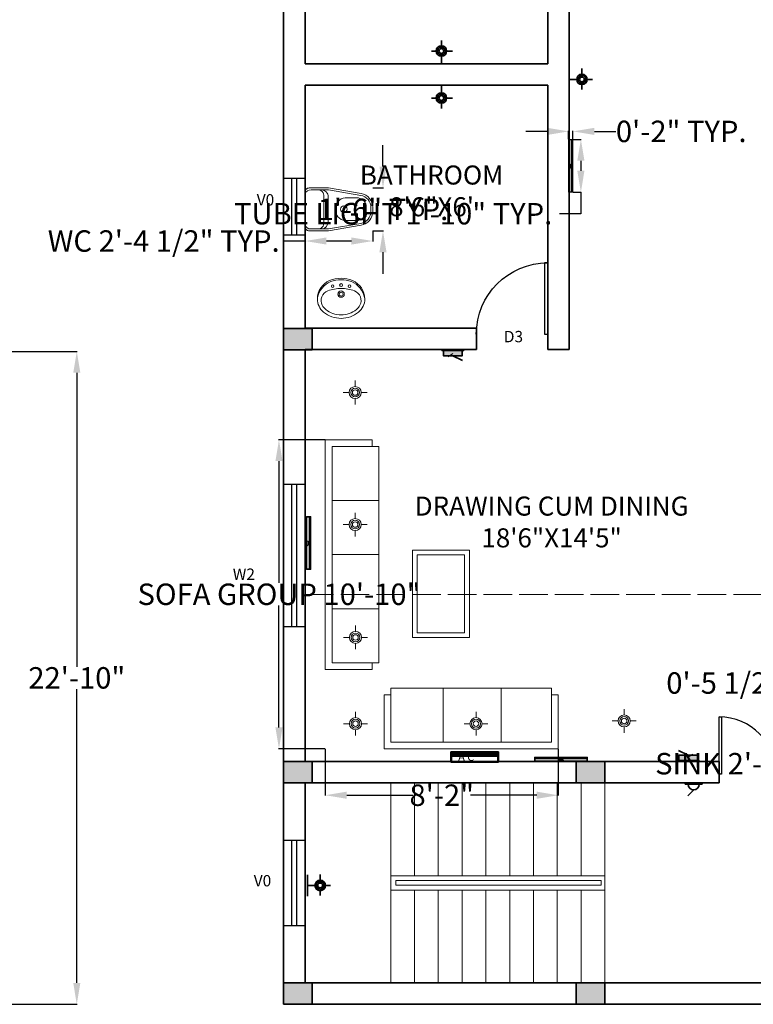
# Model space of a CAD drawing. Units: inches. Extents: x 68 to 1275, y 90 to 1276.
# Tile 4 of 6: x 608 to 916, y 603 to 1017. Entities that reach past the tile are written whole.
import ezdxf

# ---------------------------------------------------------------- set-up
doc = ezdxf.new("R2010")
doc.units = ezdxf.units.IN
doc.header["$MEASUREMENT"] = 0
doc.linetypes.add('ACAD_ISO02W100', pattern=[15, 12, -3])
for name, color, linetype, lineweight in [('A -Elec', 6, 'Continuous', 18), ('A-ANNO-TEXT', 7, 'Continuous', 18), ('A-AREA-IDEN', 7, 'Continuous', 18), ('A-FLOR-FIXT', 9, 'Continuous', 18), ('A-FURN', 150, 'Continuous', 5), ('A-WALL', 7, 'Continuous', 35), ('COLUMN', 150, 'Continuous', 35), ('DIM', 2, 'Continuous', 18), ('DOOR', 15, 'Continuous', 25), ('E-EQPM', 1, 'Continuous', 18), ('E-LITE', 6, 'Continuous', 18), ('E-POWR', 1, 'Continuous', 18), ('E-REFR', 8, 'ACAD_ISO02W100', 13), ('Elec', 1, 'Continuous', 35), ('FURN', 163, 'Continuous', 18), ('STAIRCASE', 40, 'Continuous', 18), ('WINDOW', 17, 'Continuous', 18)]:
    doc.layers.add(name, color=color, linetype=linetype, lineweight=lineweight)
doc.styles.get("Standard").update_dxf_attribs({"font": 'arial.ttf'})
doc.dimstyles.get("Standard").update_dxf_attribs({"dimtxt": 9, "dimasz": 9, "dimexe": 0.18, "dimexo": 0.0625, "dimgap": 0.09, "dimtad": 0, "dimtih": 1, "dimtoh": 1, "dimdec": 1, "dimzin": 0, "dimdsep": 46, "dimlunit": 3, "dimtxsty": 'Standard', "dimcen": 0.09, "dimadec": 0, "dimazin": 0, "dimtfac": 1, "dimtdec": 1, "dimtofl": 0, "dimtmove": 0, "dimatfit": 3, "dimfxl": 1, "dimtolj": 1, "dimtzin": 0, "dimarcsym": 0})

# ---------------------------------------------------------------- blocks, each defined once
blk = doc.blocks.new('*U2')
for p, q in [((0, 0), (0, -6)), ((40, 0), (40, -6))]:
    blk.add_line(p, q)
blk.add_lwpolyline([(0, 0), (0, 40), (1.75, 40), (1.75, 0)], close=True)
blk.add_arc((0, 0), 40, 0, 90)
blk = doc.blocks.new('W')
at = {"layer": 'DOOR'}
for p, q in [((91.84, 414.95), (100.84, 414.95)), ((91.84, 354.95), (91.84, 414.95)), ((95.34, 354.95), (95.34, 414.95)), ((97.34, 354.95), (97.34, 414.95)), ((100.84, 414.95), (100.84, 354.95)), ((100.84, 354.95), (91.84, 354.95))]:
    blk.add_line(p, q, dxfattribs=at)
blk = doc.blocks.new('V')
at = {"layer": 'DOOR'}
for p, q in [((554.81, 674.59), (563.81, 674.59)), ((554.81, 650.59), (554.81, 674.59)), ((558.31, 650.59), (558.31, 674.59)), ((560.31, 650.59), (560.31, 674.59)), ((563.81, 674.59), (563.81, 650.59)), ((563.81, 650.59), (554.81, 650.59))]:
    blk.add_line(p, q, dxfattribs=at)
blk = doc.blocks.new('W2')
at = {"layer": 'DOOR'}
for p, q in [((130.85, 208.71), (130.85, 244.71)), ((130.85, 244.71), (139.85, 244.71)), ((134.35, 208.71), (134.35, 244.71)), ((136.35, 208.71), (136.35, 244.71)), ((139.85, 244.71), (139.85, 208.71)), ((139.85, 208.71), (130.85, 208.71))]:
    blk.add_line(p, q, dxfattribs=at)
blk = doc.blocks.new('C')
h = blk.add_hatch(color=256)
h.dxf.hatch_style = 1
h.paths.add_polyline_path([(745.81, 845.98), (745.81, 857.98), (736.81, 857.98), (736.81, 845.98)])
for p, q in [((745.81, 857.98), (736.81, 857.98)), ((736.81, 857.98), (736.81, 845.98)), ((745.81, 845.98), (745.81, 857.98)), ((736.81, 845.98), (745.81, 845.98))]:
    blk.add_line(p, q)
blk = doc.blocks.new('SOFA')
at = {"layer": 'FURN'}
for p, q in [((2092.6, 1660), (2069.89, 1660)), ((2092.6, 1635.73), (2069.89, 1635.73)), ((1991.15, 1608.68), (1991.15, 1588.96)), ((2013.86, 1608.68), (2013.86, 1588.96)), ((2036.57, 1608.68), (2036.57, 1588.96))]:
    blk.add_line(p, q, dxfattribs=at)
for points in [[(2072.73, 1681.16), (2072.73, 1684), (2095.44, 1684), (2095.44, 1610.84), (2072.73, 1610.84), (2072.73, 1613.68)], [(1968.43, 1605.84), (1965.59, 1605.84), (1965.59, 1586.12), (2062.13, 1586.12), (2062.13, 1605.84), (2059.29, 1605.84)]]:
    blk.add_lwpolyline(points, dxfattribs=at)
for points in [[(2092.6, 1681.16), (2092.6, 1613.68), (2069.89, 1613.68), (2069.89, 1681.16)], [(1968.43, 1588.96), (2059.29, 1588.96), (2059.29, 1608.68), (1968.43, 1608.68)]]:
    blk.add_lwpolyline(points, close=True, dxfattribs=at)
blk = doc.blocks.new('WC')
at = {"layer": 'A-FURN'}
for p, q in [((171114.18, -56009.21), (171100.52, -56011.54)), ((171114.18, -56009.21), (171122.29, -56009.21)), ((171124.07, -56010.99), (171124.07, -56025.42)), ((171095.59, -56017.39), (171095.59, -56019.02)), ((171114.18, -56027.21), (171100.52, -56024.87)), ((171122.29, -56027.21), (171114.18, -56027.21))]:
    blk.add_line(p, q, dxfattribs=at)
for points in [[(171114.18, -56027.21), (171122.29, -56027.21, 0.414214), (171124.07, -56025.42), (171124.07, -56010.99, 0.414214), (171122.29, -56009.21), (171114.18, -56009.21), (171100.52, -56011.54, 0.365402), (171095.59, -56017.39), (171095.59, -56019.02, 0.365402), (171100.52, -56024.87)], [(171114.25, -56026.41), (171121.5, -56026.41, 0.361508), (171124.07, -56024.7), (171124.07, -56011.71, 0.375474), (171121.68, -56010), (171114.25, -56010), (171100.66, -56012.32, 0.365402), (171096.38, -56017.39), (171096.38, -56019.02, 0.365402), (171100.66, -56024.09)], [(171124.07, -56011.71), (171124.07, -56024.7, -0.361508), (171121.5, -56026.41), (171117.23, -56026.41, -0.430105), (171114.38, -56023.46), (171114.38, -56012.95, -0.411531), (171117.23, -56010), (171121.68, -56010, -0.375474)], [(171124.07, -56011.71), (171124.07, -56024.7, -0.361508), (171121.5, -56026.41), (171118.83, -56026.41, -0.480412), (171116.16, -56023.63), (171116.16, -56012.78, -0.482705), (171118.83, -56010), (171121.68, -56010, -0.375474)], [(171106.42, -56023.02, 0.46477), (171111.04, -56019.12), (171111.04, -56017.49, 0.46477), (171106.42, -56013.59), (171101.64, -56013.59, 0.365402), (171098.35, -56017.49), (171098.35, -56019.12, 0.365402), (171101.64, -56023.02)], [(171107.8, -56016.9, -1), (171107.8, -56019.71, -1)]]:
    blk.add_lwpolyline(points, format="xyb", close=True, dxfattribs=at)
for centre, radius, start, end in [((171101.52, -56017.39), 5.93, 99.7106, 180.0002), ((171122.29, -56010.99), 1.78, 0.0002, 90.0002), ((171101.52, -56019.02), 5.93, 180.0002, 260.2897), ((171122.29, -56025.42), 1.78, 270.0002, 0.0002)]:
    blk.add_arc(centre, radius, start, end, dxfattribs=at)
blk = doc.blocks.new('Basin')
at = {"layer": 'A-FURN'}
for centre, radius in [((171010.96, -56068.51), 0.593), ((171010.45, -56072.47), 0.692), ((171014.68, -56072.47), 1.48), ((171014.68, -56072.47), 0.91), ((171010.96, -56076.42), 0.593)]:
    blk.add_circle(centre, radius, dxfattribs=at)
for centre, radius, start, end in [((171018.29, -56073.43), 10.2, 262.5047, 262.5047), ((171016.96, -56070.69), 9.3, 90, 157.2856), ((171018.29, -56071.51), 10.2, 100.9967, 157.8207), ((171017.65, -56067.95), 4.81, 62.931, 159.6415), ((171016.96, -56069.3), 7.91, 39.0829, 90), ((171016.96, -56069.3), 6.33, 39.0829, 62.931), ((171013.06, -56072.47), 12.93, 0, 39.0829), ((171021.21, -56072.47), 13.91, 157.2856, 180), ((171021.21, -56072.47), 13.27, 158.7467, 180), ((171029.84, -56072.47), 17.8, 159.6415, 180), ((171013.06, -56072.47), 11.35, 0, 39.0829), ((171021.21, -56072.47), 13.91, 180, 202.7144), ((171021.21, -56072.47), 13.27, 180, 201.2533), ((171029.84, -56072.47), 17.8, 180, 200.3585), ((171013.06, -56072.47), 11.35, 320.9171, 0), ((171013.06, -56072.47), 12.93, 320.9171, 0), ((171016.96, -56074.25), 9.3, 202.7144, 270), ((171018.29, -56073.43), 10.2, 202.1793, 259.0033), ((171017.65, -56076.99), 4.81, 200.3585, 297.069), ((171016.96, -56075.63), 7.91, 270, 320.9171), ((171016.96, -56075.63), 6.33, 297.069, 320.9171)]:
    blk.add_arc(centre, radius, start, end, dxfattribs=at)
blk = doc.blocks.new('splight')
at = {"layer": 'Elec'}
for p, q in [((4618.17, 527.16), (4627.57, 527.16)), ((4622.87, 527.16), (4622.87, 523.87)), ((4620.58, 521.58), (4618.05, 521.58)), ((4625.16, 521.58), (4627.23, 521.58)), ((4622.87, 519.28), (4622.87, 517.03))]:
    blk.add_line(p, q, dxfattribs=at)
for radius in [2.29, 1.67, 1.04]:
    blk.add_circle((4622.87, 521.58), radius, dxfattribs=at)
blk = doc.blocks.new('tube')
at = {"layer": 'A -Elec'}
for p, q in [((4592.61, 556.75), (4641.61, 556.75)), ((4592.61, 555.25), (4592.61, 556.75)), ((4593.11, 555.25), (4593.11, 556.75)), ((4593.11, 556.33), (4593.41, 556.33)), ((4593.41, 555.25), (4593.41, 556.75)), ((4593.41, 556.5), (4640.81, 556.5)), ((4640.81, 555.25), (4640.81, 556.75)), ((4640.81, 556.33), (4641.11, 556.33)), ((4641.11, 556.75), (4641.11, 555.25)), ((4641.11, 555.25), (4641.11, 556.75)), ((4641.61, 556.75), (4641.61, 555.25)), ((4592.61, 552.75), (4592.61, 555.25)), ((4592.61, 552.75), (4641.61, 552.75)), ((4593.11, 556.21), (4593.41, 556.21)), ((4593.11, 555.81), (4593.41, 555.81)), ((4593.11, 555.69), (4593.41, 555.69)), ((4641.11, 555.25), (4593.11, 555.25)), ((4593.11, 555.25), (4593.11, 553.25)), ((4593.11, 553.25), (4593.11, 555.25)), ((4593.11, 553.25), (4641.61, 553.25)), ((4593.41, 556.25), (4640.81, 556.25)), ((4593.41, 556), (4640.81, 556)), ((4593.41, 555.75), (4640.81, 555.75)), ((4593.41, 555.5), (4640.81, 555.5)), ((4640.81, 556.21), (4641.11, 556.21)), ((4640.81, 555.81), (4641.11, 555.81)), ((4640.81, 555.69), (4641.11, 555.69)), ((4641.11, 553.25), (4641.11, 555.25)), ((4641.61, 552.75), (4641.61, 555.25))]:
    blk.add_line(p, q, dxfattribs=at)
for points in [[(4615.6, 553.25), (4619.11, 553.25), (4619.11, 554.31), (4615.6, 554.31)], [(4619.11, 553.78), (4619.11, 553.78), (4619.11, 553.78), (4619.11, 553.78)], [(4619.11, 553.78), (4619.81, 553.78), (4619.81, 553.25), (4619.11, 553.25)]]:
    blk.add_lwpolyline(points, close=True, dxfattribs=at)
blk = doc.blocks.new('CIELING')
at = {"layer": 'A -Elec'}
for p, q in [((1070.87, -8395.66), (1070.87, -8391.49)), ((1066.61, -8399.91), (1062.44, -8399.91)), ((1075.13, -8399.91), (1079.29, -8399.91)), ((1070.87, -8408.34), (1070.87, -8404.17))]:
    blk.add_line(p, q, dxfattribs=at)
for radius in [4.26, 3.1, 1.94]:
    blk.add_circle((1070.87, -8399.91), radius, dxfattribs=at)
blk = doc.blocks.new('BELL SWITCH')
at = {"layer": 'Elec'}
for p, q in [((4981.81, 3401.31), (4981.81, 3402.27)), ((4981.81, 3402.27), (4993.57, 3402.27)), ((4993.57, 3402.27), (4993.57, 3401.31)), ((4993.57, 3401.31), (4981.81, 3401.31)), ((4987.69, 3397.36), (4983.52, 3393.3))]:
    blk.add_line(p, q, dxfattribs=at)
blk.add_arc((4987.69, 3401.31), 3.95, 180, 0, dxfattribs=at)
blk = doc.blocks.new('ac')
at = {"layer": 'Elec'}
for p, q in [((12718.34, -53.78), (12674.36, -53.78)), ((12674.36, -63.02), (12674.36, -53.78)), ((12675.81, -57.52), (12675.81, -53.78)), ((12717.03, -57.52), (12717.03, -53.78)), ((12718.34, -63.02), (12718.34, -53.78)), ((12718.34, -63.02), (12674.36, -63.02)), ((12674.89, -57.52), (12717.81, -57.52)), ((12717.03, -54.85), (12675.81, -54.85)), ((12717.03, -56.21), (12675.81, -56.21))]:
    blk.add_line(p, q, dxfattribs=at)
at = {"layer": 'Elec', "ltscale": 0.1}
for p, q in [((12674.89, -61.49), (12674.89, -53.78)), ((12717.03, -54.36), (12675.81, -54.36)), ((12717.81, -61.49), (12717.81, -53.78)), ((12717.03, -55.66), (12675.81, -55.66)), ((12717.03, -56.84), (12675.81, -56.84)), ((12716.81, -62.49), (12675.89, -62.49))]:
    blk.add_line(p, q, dxfattribs=at)
at = {"layer": 'Elec'}
for centre, start, end in [((12675.89, -61.49), 180, 270), ((12716.81, -61.49), 270, 0)]:
    blk.add_arc(centre, 1, start, end, dxfattribs=at)
blk = doc.blocks.new('STAIR-RETURN-PLAN')
for p, q in [((0, 84), (0, 0)), ((10, 84), (10, 45)), ((20, 84), (20, 45)), ((30, 84), (30, 45)), ((40, 84), (40, 45)), ((50, 84), (50, 45)), ((60, 84), (60, 45)), ((70, 84), (70, 45)), ((80, 84), (80, 45)), ((90, 84), (90, 0)), ((0, 45), (90, 45)), ((2.15, 43), (88.44, 43)), ((2.15, 41), (2.15, 43)), ((88.44, 41), (88.44, 43)), ((0, 39), (90, 39)), ((2.15, 41), (88.44, 41)), ((10, 39), (10, 0)), ((20, 39), (20, 0)), ((30, 39), (30, 0)), ((40, 39), (40, 0)), ((50, 39), (50, 0)), ((60, 39), (60, 0)), ((70, 39), (70, 0)), ((80, 39), (80, 0))]:
    blk.add_line(p, q)
blk = doc.blocks.new('elec box')
at = {"layer": 'Elec'}
blk.add_hatch(color=256, dxfattribs=at).paths.add_polyline_path([(3828.23, 599.29), (3828.23, 594.79), (3844.73, 594.79), (3844.73, 599.29)])
for p, q in [((3836.48, 599.29), (3828.07, 603.45)), ((3846.1, 594.79), (3826.83, 594.79)), ((3826.83, 594.79), (3826.83, 593.89)), ((3846.1, 593.89), (3846.1, 594.79)), ((3826.83, 593.89), (3846.1, 593.89))]:
    blk.add_line(p, q, dxfattribs=at)
blk.add_lwpolyline([(3828.23, 594.79), (3828.23, 599.29), (3844.73, 599.29), (3844.73, 594.79), (3828.23, 594.79)], dxfattribs=at)
blk = doc.blocks.new('SWITCHBOARD-ONE-WAY')
blk.add_line((4.63, 1.73), (6.64, 3.12))
at = {"xscale": 0.480395109260985, "yscale": 0.480395109260985, "zscale": 0.480395109260985}
blk.add_blockref('elec box', (-1838.39, -285.3), dxfattribs=at)
blk = doc.blocks.new('*D59')
at = {"layer": 'Defpoints', "color": 0, "transparency": 16777216}
for p in [(727.63, 928.31), (756.11, 928.31), (727.63, 924.04)]:
    blk.add_point(p, dxfattribs=at)
at = {"layer": 'DIM', "color": 0, "lineweight": -2, "transparency": 16777216}
for p, q in [((727.63, 928.25), (727.63, 923.86)), ((756.11, 928.25), (756.11, 923.86)), ((727.63, 924.04), (718.63, 924.04)), ((747.11, 924.04), (736.63, 924.04))]:
    blk.add_line(p, q, dxfattribs=at)
at = {"layer": 'DIM', "color": 0, "transparency": 16777216}
for points in [[(736.63, 925.54), (736.63, 922.54), (727.63, 924.04)], [(747.11, 925.54), (747.11, 922.54), (756.11, 924.04)]]:
    blk.add_solid(points, dxfattribs=at)
at = {"layer": 'DIM', "color": 0, "transparency": 16777216, "insert": (668.22, 924.04), "char_height": 9, "attachment_point": 5}
blk.add_mtext('\\A1;WC 2\'-4 1/2" TYP.', dxfattribs=at)
blk = doc.blocks.new('*D60')
at = {"layer": 'Defpoints', "color": 0, "transparency": 16777216}
for p in [(756.11, 946.31), (756.11, 928.31), (760.38, 928.31)]:
    blk.add_point(p, dxfattribs=at)
at = {"layer": 'DIM', "color": 0, "lineweight": -2, "transparency": 16777216}
for p, q in [((760.38, 955.31), (760.38, 964.31)), ((756.17, 946.31), (760.56, 946.31)), ((756.17, 928.31), (760.56, 928.31)), ((760.38, 919.31), (760.38, 910.31))]:
    blk.add_line(p, q, dxfattribs=at)
at = {"layer": 'DIM', "color": 0, "transparency": 16777216}
for points in [[(758.88, 955.31), (761.88, 955.31), (760.38, 946.31)], [(758.88, 919.31), (761.88, 919.31), (760.38, 928.31)]]:
    blk.add_solid(points, dxfattribs=at)
at = {"layer": 'DIM', "color": 0, "transparency": 16777216, "insert": (760.38, 937.31), "char_height": 9, "attachment_point": 5}
blk.add_mtext('\\A1;1\'-6" TYP.', dxfattribs=at)
blk = doc.blocks.new('*D63')
at = {"layer": 'Defpoints', "color": 0, "transparency": 16777216}
for p in [(736.14, 840.6), (716.66, 710.75), (736.14, 710.75)]:
    blk.add_point(p, dxfattribs=at)
at = {"layer": 'DIM', "color": 0, "lineweight": -2, "transparency": 16777216}
for p, q in [((736.07, 840.6), (716.48, 840.6)), ((716.66, 831.6), (716.66, 780.43)), ((716.66, 719.75), (716.66, 770.93)), ((736.07, 710.75), (716.48, 710.75))]:
    blk.add_line(p, q, dxfattribs=at)
at = {"layer": 'DIM', "color": 0, "transparency": 16777216}
for points in [[(715.16, 831.6), (718.16, 831.6), (716.66, 840.6)], [(715.16, 719.75), (718.16, 719.75), (716.66, 710.75)]]:
    blk.add_solid(points, dxfattribs=at)
at = {"layer": 'DIM', "color": 0, "transparency": 16777216, "insert": (716.66, 775.68), "char_height": 9, "attachment_point": 5}
blk.add_mtext('\\A1;SOFA GROUP 10\'-10"', dxfattribs=at)
blk = doc.blocks.new('*D64')
at = {"layer": 'Defpoints', "color": 0, "transparency": 16777216}
for p in [(736.14, 710.75), (834.01, 710.75), (834.01, 691.28)]:
    blk.add_point(p, dxfattribs=at)
at = {"layer": 'DIM', "color": 0, "lineweight": -2, "transparency": 16777216}
for p, q in [((736.14, 710.69), (736.14, 691.1)), ((834.01, 710.69), (834.01, 691.1)), ((745.14, 691.28), (773.02, 691.28)), ((825.01, 691.28), (797.13, 691.28))]:
    blk.add_line(p, q, dxfattribs=at)
at = {"layer": 'DIM', "color": 0, "transparency": 16777216}
for points in [[(745.14, 692.78), (745.14, 689.78), (736.14, 691.28)], [(825.01, 692.78), (825.01, 689.78), (834.01, 691.28)]]:
    blk.add_solid(points, dxfattribs=at)
at = {"layer": 'DIM', "color": 0, "transparency": 16777216, "insert": (785.08, 691.28), "char_height": 9, "attachment_point": 5}
blk.add_mtext('\\A1;8\'-2"', dxfattribs=at)
blk = doc.blocks.new('*D68')
at = {"layer": 'Defpoints', "color": 0, "transparency": 16777216}
for p in [(944.14, 747.41), (949.63, 747.41), (944.14, 738.41)]:
    blk.add_point(p, dxfattribs=at)
at = {"layer": 'DIM', "color": 0, "lineweight": -2, "transparency": 16777216}
for p, q in [((944.14, 747.35), (944.14, 738.23)), ((949.63, 747.35), (949.63, 738.23)), ((935.14, 738.41), (926.14, 738.41)), ((958.63, 738.41), (967.63, 738.41))]:
    blk.add_line(p, q, dxfattribs=at)
at = {"layer": 'DIM', "color": 0, "transparency": 16777216}
for points in [[(935.14, 739.91), (935.14, 736.91), (944.14, 738.41)], [(958.63, 739.91), (958.63, 736.91), (949.63, 738.41)]]:
    blk.add_solid(points, dxfattribs=at)
at = {"layer": 'DIM', "color": 0, "transparency": 16777216, "insert": (903.6, 738.41), "char_height": 9, "attachment_point": 5}
blk.add_mtext('\\A1;0\'-5 1/2"', dxfattribs=at)
blk = doc.blocks.new('*D69')
at = {"layer": 'Defpoints', "color": 0, "transparency": 16777216}
for p in [(962.08, 709.07), (992.43, 709.07), (962.08, 704.52)]:
    blk.add_point(p, dxfattribs=at)
at = {"layer": 'DIM', "color": 0, "lineweight": -2, "transparency": 16777216}
for p, q in [((962.08, 709.01), (962.08, 704.34)), ((992.43, 709.01), (992.43, 704.34)), ((962.08, 704.52), (953.08, 704.52)), ((983.43, 704.52), (971.08, 704.52))]:
    blk.add_line(p, q, dxfattribs=at)
at = {"layer": 'DIM', "color": 0, "transparency": 16777216}
for points in [[(971.08, 706.02), (971.08, 703.02), (962.08, 704.52)], [(983.43, 706.02), (983.43, 703.02), (992.43, 704.52)]]:
    blk.add_solid(points, dxfattribs=at)
at = {"layer": 'DIM', "color": 0, "transparency": 16777216, "insert": (914.15, 704.52), "char_height": 9, "attachment_point": 5}
blk.add_mtext('\\A1;SINK 2\'-6 1/2"', dxfattribs=at)
blk = doc.blocks.new('*D75')
at = {"layer": 'Defpoints', "color": 0, "transparency": 16777216}
for p in [(840.21, 966.74), (840.21, 944.52), (843.55, 944.52)]:
    blk.add_point(p, dxfattribs=at)
at = {"layer": 'DIM', "color": 0, "lineweight": -2, "transparency": 16777216}
for p, q in [((840.28, 966.74), (843.73, 966.74)), ((843.55, 957.74), (843.55, 953.52)), ((840.28, 944.52), (843.73, 944.52)), ((843.55, 944.52), (843.55, 935.52)), ((843.55, 935.52), (834.55, 935.52))]:
    blk.add_line(p, q, dxfattribs=at)
at = {"layer": 'DIM', "color": 0, "transparency": 16777216}
for points in [[(842.05, 957.74), (845.05, 957.74), (843.55, 966.74)], [(842.05, 953.52), (845.05, 953.52), (843.55, 944.52)]]:
    blk.add_solid(points, dxfattribs=at)
at = {"layer": 'DIM', "color": 0, "transparency": 16777216, "insert": (764.65, 935.52), "char_height": 9, "attachment_point": 5}
blk.add_mtext('\\A1;TUBE LIGHT 1\'-10" TYP.', dxfattribs=at)
blk = doc.blocks.new('*D76')
at = {"layer": 'Defpoints', "color": 0, "transparency": 16777216}
for p in [(840.21, 970.08), (838.4, 966.74), (840.21, 966.74)]:
    blk.add_point(p, dxfattribs=at)
at = {"layer": 'DIM', "color": 0, "lineweight": -2, "transparency": 16777216}
for p, q in [((829.4, 970.08), (820.4, 970.08)), ((838.4, 966.81), (838.4, 970.26)), ((840.21, 966.81), (840.21, 970.26)), ((849.21, 970.08), (858.21, 970.08))]:
    blk.add_line(p, q, dxfattribs=at)
at = {"layer": 'DIM', "color": 0, "transparency": 16777216}
for points in [[(829.4, 971.58), (829.4, 968.58), (838.4, 970.08)], [(849.21, 971.58), (849.21, 968.58), (840.21, 970.08)]]:
    blk.add_solid(points, dxfattribs=at)
at = {"layer": 'DIM', "color": 0, "transparency": 16777216, "insert": (885.73, 970.08), "char_height": 9, "attachment_point": 5}
blk.add_mtext('\\A1;0\'-2" TYP.', dxfattribs=at)
blk = doc.blocks.new('*D84')
at = {"layer": 'Defpoints', "color": 0, "transparency": 16777216}
for p in [(594.19, 877.68), (631.69, 877.68), (534.19, 603.47)]:
    blk.add_point(p, dxfattribs=at)
at = {"layer": 'DIM', "color": 0, "lineweight": -2, "transparency": 16777216}
for p, q in [((594.25, 877.68), (631.87, 877.68)), ((631.69, 868.68), (631.69, 745.26)), ((631.69, 612.47), (631.69, 735.89)), ((534.25, 603.47), (631.87, 603.47))]:
    blk.add_line(p, q, dxfattribs=at)
at = {"layer": 'DIM', "color": 0, "transparency": 16777216}
for points in [[(630.19, 868.68), (633.19, 868.68), (631.69, 877.68)], [(630.19, 612.47), (633.19, 612.47), (631.69, 603.47)]]:
    blk.add_solid(points, dxfattribs=at)
at = {"layer": 'DIM', "color": 0, "transparency": 16777216, "insert": (631.69, 740.57), "char_height": 9, "attachment_point": 5}
blk.add_mtext('\\A1;22\'-10"', dxfattribs=at)
blk = doc.blocks.new('*D112')
at = {"layer": 'Defpoints', "color": 0, "transparency": 16777216}
for p in [(1147.63, 1270.42), (718.63, 1232.47), (1147.63, 988.68)]:
    blk.add_point(p, dxfattribs=at)
at = {"layer": 'DIM', "color": 0, "lineweight": -2, "transparency": 16777216}
for p, q in [((718.63, 1232.53), (718.63, 1270.6)), ((727.63, 1270.42), (917.58, 1270.42)), ((1138.63, 1270.42), (948.67, 1270.42)), ((1147.63, 988.74), (1147.63, 1270.6))]:
    blk.add_line(p, q, dxfattribs=at)
at = {"layer": 'DIM', "color": 0, "transparency": 16777216}
for points in [[(727.63, 1271.92), (727.63, 1268.92), (718.63, 1270.42)], [(1138.63, 1271.92), (1138.63, 1268.92), (1147.63, 1270.42)]]:
    blk.add_solid(points, dxfattribs=at)
at = {"layer": 'DIM', "color": 0, "transparency": 16777216, "insert": (933.13, 1270.42), "char_height": 9, "attachment_point": 5}
blk.add_mtext('\\A1;35\'-9"', dxfattribs=at)

msp = doc.modelspace()

# ---------------------------------------------------------------- linework, layer by layer
at = {"layer": 'A-WALL'}
for p, q in [((718.63, 1232.47), (718.63, 603.47)), ((727.63, 1082.47), (727.63, 998.47)), ((829.63, 1082.47), (829.63, 998.47)), ((838.63, 1082.47), (838.63, 986.47)), ((727.63, 998.47), (829.63, 998.47)), ((727.63, 989.47), (829.63, 989.47)), ((727.63, 989.47), (727.63, 887.47)), ((829.63, 989.47), (829.63, 887.47)), ((838.63, 986.47), (838.63, 878.47)), ((727.63, 887.47), (799.63, 887.47)), ((799.63, 887.47), (799.63, 878.47)), ((829.63, 887.47), (829.63, 878.47)), ((727.63, 878.47), (799.63, 878.47)), ((727.63, 878.47), (727.63, 705.47)), ((829.63, 878.47), (838.63, 878.47)), ((727.63, 705.47), (901.63, 705.47)), ((901.63, 696.47), (901.63, 705.47)), ((727.63, 696.47), (901.63, 696.47)), ((727.63, 696.47), (727.63, 612.47)), ((727.63, 612.47), (949.63, 612.47)), ((718.63, 603.47), (1087.63, 603.47))]:
    msp.add_line(p, q, dxfattribs=at)
at = {"layer": 'E-REFR'}
msp.add_line((727.63, 775.56), (949.63, 775.56), dxfattribs=at)
at = {"layer": 'FURN'}
for points in [[(796.69, 757.54), (772.77, 757.54), (772.77, 794.24), (796.69, 794.24)], [(794.69, 759.54), (774.77, 759.54), (774.77, 792.24), (794.69, 792.24)]]:
    msp.add_lwpolyline(points, close=True, dxfattribs=at)

# ---------------------------------------------------------------- block references
at = {"layer": 'A-FLOR-FIXT', "rotation": 180}
msp.add_blockref('WC', (171851.7, -55080.89), dxfattribs=at)
at = {"layer": 'A-FLOR-FIXT', "ltscale": 0.05, "xscale": 0.900000000023283, "yscale": 0.900000000023283, "zscale": 0.900000000023283, "rotation": 270}
msp.add_blockref('Basin', (51207.99, 154814.94), dxfattribs=at)
at = {"layer": 'COLUMN', "rotation": 270}
for p in [(-127.36, 1624.13), (-127.36, 1442.31), (-4.36, 1442.28), (-127.36, 1349.28), (-4.36, 1349.28)]:
    msp.add_blockref('C', p, dxfattribs=at)
at = {"layer": 'DOOR'}
for p, xscale, yscale, zscale in [((829.63, 884.85), -0.7506967006010635, 0.7506967006010635, 0.7506967006010635), ((901.63, 700.08), 0.6023265859053817, 0.6023265859053817, 0.6023265859053817)]:
    msp.add_blockref('*U2', p, dxfattribs=dict(at, xscale=xscale, yscale=yscale, zscale=zscale))
at = {"layer": 'E-EQPM', "xscale": 0.4550488862921059, "yscale": 0.4550488862921059, "zscale": 0.4550488862921059}
msp.add_blockref('ac', (-4978.55, 733.91), dxfattribs=at)
at = {"layer": 'E-LITE', "yscale": 0.9617510087435096, "zscale": 0.9617510087390623}
for p, xscale, rotation in [((5230.97, 1505.46), 0.9617510087435096, 180.0000000000001), ((1345.62, 5437.96), -0.9617510087435096, 89.99999999999976), ((5230.97, 482.47), -0.9617510087435096, 359.9999999999997), ((1235.61, 5099.43), -0.9617510087435096, 89.99999999999976)]:
    msp.add_blockref('splight', p, dxfattribs=dict(at, xscale=xscale, rotation=rotation))
at = {"layer": 'E-LITE', "transparency": 33554676, "xscale": 0.4534687213066354, "yscale": 0.4534687213066354, "zscale": 0.4534687213066354, "rotation": 270}
for p in [(587.74, 3049.35), (477.53, 2890.96)]:
    msp.add_blockref('tube', p, dxfattribs=at)
at = {"layer": 'E-LITE', "transparency": 33554676}
for name, p, xscale, yscale, zscale in [('CIELING', (113.61, 5841.99), 0.5930528030907906, 0.5930528030907906, 0.5930528030907906), ('CIELING', (113.61, 5786.54), 0.5930528030907906, 0.5930528030907906, 0.5930528030907906), ('CIELING', (113.75, 5739.15), 0.5930528030907906, 0.5930528030907906, 0.5930528030907906), ('CIELING', (113.75, 5702.92), 0.5930528030907906, 0.5930528030907906, 0.5930528030907906), ('CIELING', (164.39, 5702.92), 0.5930528030907906, 0.5930528030907906, 0.5930528030907906), ('CIELING', (226.67, 5704.07), 0.5930528030907906, 0.5930528030907906, 0.5930528030907906), ('tube', (-1258.55, 454.81), 0.4534687213066354, 0.4534687213066354, 0.4534687213066354)]:
    msp.add_blockref(name, p, dxfattribs=dict(at, xscale=xscale, yscale=yscale, zscale=zscale))
at = {"layer": 'E-POWR', "rotation": 180}
msp.add_blockref('SWITCHBOARD-ONE-WAY', (794.35, 878.47), dxfattribs=at)
at = {"layer": 'E-POWR'}
msp.add_blockref('SWITCHBOARD-ONE-WAY', (884.03, 705.47), dxfattribs=at)
at = {"layer": 'E-POWR', "xscale": 0.6004938865802444, "yscale": 0.6004938865802444, "zscale": 0.6004938865802444}
msp.add_blockref('BELL SWITCH', (-2104.12, -1346.57), dxfattribs=at)
at = {"layer": 'FURN', "rotation": 270}
msp.add_blockref('SOFA', (-849.99, 2806.2), dxfattribs=at)
at = {"layer": 'STAIRCASE'}
msp.add_blockref('STAIR-RETURN-PLAN', (763.63, 612.47), dxfattribs=at)
at = {"layer": 'WINDOW'}
for name, p in [('V', (163.82, 275.88)), ('W', (626.79, 407.02)), ('W2', (587.77, 427.75))]:
    msp.add_blockref(name, p, dxfattribs=at)

# ---------------------------------------------------------------- texts
at = {"layer": 'A-ANNO-TEXT', "char_height": 5.9531, "width": 20.3989, "attachment_point": 5}
for s, insert in [('{\\fTimes New Roman|b0|i0|c0|p18;\\H0.8x;V0}', (710.99, 941.34)), ('{\\fTimes New Roman|b0|i0|c0|p18;\\H0.8x;D3}', (815.21, 883.9)), ('{\\fTimes New Roman|b0|i0|c0|p18;\\H0.8x;W2}', (701.91, 784.12)), ('{\\fTimes New Roman|b0|i0|c0|p18;\\H0.8x;V0}', (709.73, 655.37))]:
    msp.add_mtext(s, dxfattribs=dict(at, insert=insert))
at = {"layer": 'A-AREA-IDEN', "char_height": 8, "attachment_point": 2}
for s, insert in [('BATHROOM\\P8\'6"X6\'', (780.8, 955.76)), ('DRAWING CUM DINING\\P18\'6"X14\'5"', (831.26, 816.71))]:
    msp.add_mtext_dynamic_manual_height_columns(s, width=128.8568, gutter_width=1, heights=[0], dxfattribs=dict(at, insert=insert))
at = {"layer": 'E-EQPM'}
msp.add_text(' A C', height=3.363, dxfattribs=at).set_placement((790.96, 705.7))

# ---------------------------------------------------------------- dimensions: what is measured, and where the dimension line sits
at = {"layer": 'DIM'}
for base, p1, p2, picture, middle in [((1147.63, 1270.42), (718.63, 1232.47), (1147.63, 988.68), '*D112', (933.13, 1270.42)), ((834.01, 691.28), (736.14, 710.75), (834.01, 710.75), '*D64', (785.08, 691.28))]:
    dim = msp.add_linear_dim(base=base, p1=p1, p2=p2, dimstyle='Standard', override={"dimdec": 1, "dimlfac": 1, "dimrnd": 0, "dimzin": 1, "dimdsep": 46, "dimlunit": 4, "dimfrac": 2}, dxfattribs=at)
    dim.commit()
    dim.dimension.update_dxf_attribs({"geometry": picture, "text_midpoint": middle})
dim = msp.add_linear_dim(base=(840.21, 970.08), p1=(838.4, 966.74), p2=(840.21, 966.74), text='<> TYP.', dimstyle='Standard', override={"dimdec": 1, "dimlfac": 1, "dimrnd": 0, "dimzin": 1, "dimdsep": 46, "dimlunit": 4, "dimfrac": 2}, dxfattribs=at)
dim.commit()
dim.dimension.update_dxf_attribs({"geometry": '*D76', "text_midpoint": (885.73, 970.08)})
for base, p1, p2, angle, text, picture, middle in [((843.55, 944.52), (840.21, 966.74), (840.21, 944.52), 270, 'TUBE LIGHT <> TYP.', '*D75', (764.65, 935.52)), ((760.38, 928.31), (756.11, 946.31), (756.11, 928.31), 270, '<> TYP.', '*D60', (760.38, 937.31)), ((727.63, 924.04), (756.11, 928.31), (727.63, 928.31), 180, 'WC <> TYP.', '*D59', (668.22, 924.04)), ((716.6593, 710.7549), (736.1366, 840.603), (736.1366, 710.7549), 270, 'SOFA GROUP <>', '*D63', (716.6593, 775.6789)), ((962.0814, 704.5209), (992.4312, 709.0734), (962.0814, 709.0734), 180, 'SINK <>', '*D69', (914.1459, 704.5209))]:
    dim = msp.add_linear_dim(base=base, p1=p1, p2=p2, angle=angle, text=text, dimstyle='Standard', override={"dimdec": 1, "dimlfac": 1, "dimrnd": 0, "dimzin": 1, "dimdsep": 46, "dimlunit": 4, "dimfrac": 2}, dxfattribs=at)
    dim.commit()
    dim.dimension.update_dxf_attribs({"geometry": picture, "text_midpoint": middle})
for base, p1, p2, angle, picture, middle in [((631.69, 877.68), (534.19, 603.47), (594.19, 877.68), 90, '*D84', (631.69, 740.57)), ((944.14, 738.41), (949.63, 747.41), (944.14, 747.41), 180, '*D68', (903.6, 738.41))]:
    dim = msp.add_linear_dim(base=base, p1=p1, p2=p2, angle=angle, dimstyle='Standard', override={"dimdec": 1, "dimlfac": 1, "dimrnd": 0, "dimzin": 1, "dimdsep": 46, "dimlunit": 4, "dimfrac": 2}, dxfattribs=at)
    dim.commit()
    dim.dimension.update_dxf_attribs({"geometry": picture, "text_midpoint": middle})

doc.saveas('drawing.dxf')
